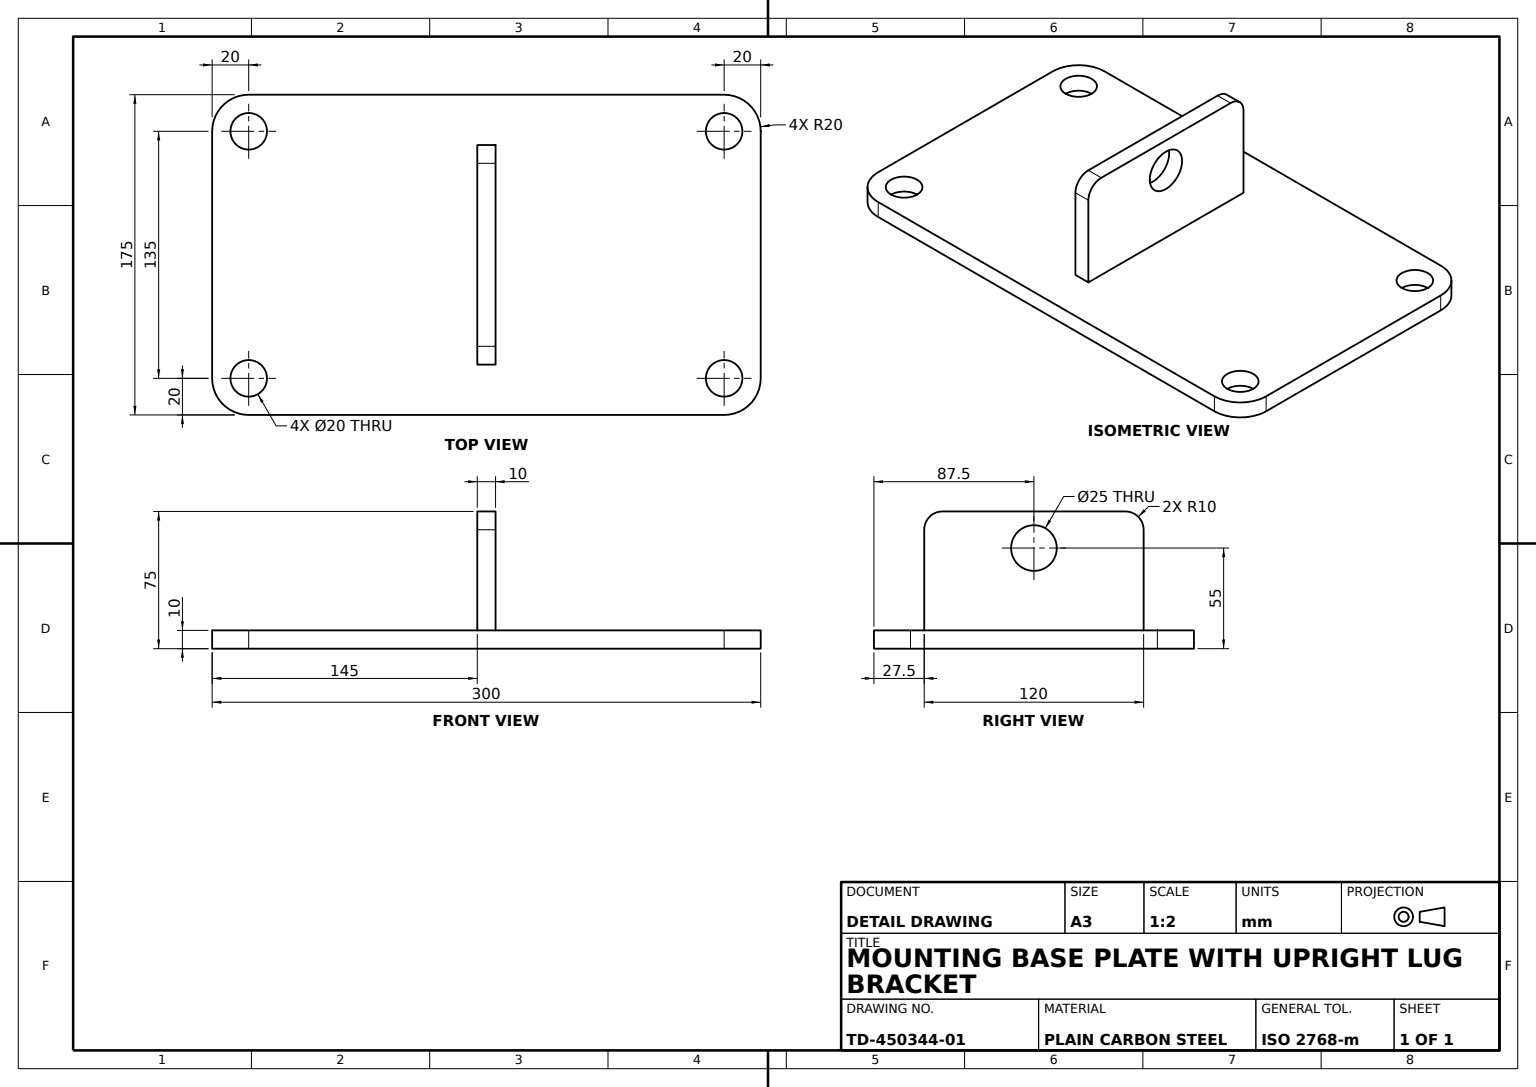
from build123d import *

# Parameters (mm, degrees)
BASE_PLATE_DEPTH          = 10
MOUNTING_HOLES_SKETCH_R   = 10
MOUNTING_HOLES_4X_DEPTH   = 10
UPRIGHT_TAB_SKETCH_W      = 10
UPRIGHT_TAB_SKETCH_H      = 120
UPRIGHT_TAB_DEPTH         = 65
TAB_CORNER_FILLET_1_R10_R = 10
TAB_CORNER_FILLET_2_R10_R = 10
TAB_HOLE_SKETCH_R         = 12.5
TAB_HOLE_DEPTH            = 65


with BuildPart() as part:
    # Base Plate Sketch → Base Plate (new body)
    with BuildSketch(Plane(origin=(0, 0, 0), x_dir=(1, 0, 0), z_dir=(0, 1, 0))):
        with BuildLine():
            Line((-130, -87.5), (130, -87.5))
            ThreePointArc((130, -87.5), (144.142135624, -81.642135624), (150, -67.5))
            Line((150, -67.5), (150, 67.5))
            ThreePointArc((150, 67.5), (144.142135624, 81.642135624), (130, 87.5))
            Line((130, 87.5), (-130, 87.5))
            ThreePointArc((-130, 87.5), (-144.142135624, 81.642135624), (-150, 67.5))
            Line((-150, 67.5), (-150, -67.5))
            ThreePointArc((-150, -67.5), (-144.142135624, -81.642135624), (-130, -87.5))
        make_face()
    extrude(amount=BASE_PLATE_DEPTH)

    # Mounting Holes Sketch → Mounting Holes 4x (cut)
    with BuildSketch(Plane(origin=(0, 10, 0), x_dir=(1, 0, 0), z_dir=(0, 1, 0))):
        with Locations(Location((130, 67.5, 0), (0, 0, 270))):
            Circle(MOUNTING_HOLES_SKETCH_R)
        with Locations(Location((130, -67.5, 0), (0, 0, 270))):
            Circle(MOUNTING_HOLES_SKETCH_R)
        with Locations(Location((-130, 67.5, 0), (0, 0, 270))):
            Circle(MOUNTING_HOLES_SKETCH_R)
        with Locations(Location((-130, -67.5, 0), (0, 0, 270))):
            Circle(MOUNTING_HOLES_SKETCH_R)
    extrude(amount=-MOUNTING_HOLES_4X_DEPTH, mode=Mode.SUBTRACT)

    # Upright Tab Sketch → Upright Tab (add)
    with BuildSketch(Plane(origin=(0, 10, 0), x_dir=(1, 0, 0), z_dir=(0, 1, 0))):
        Rectangle(UPRIGHT_TAB_SKETCH_W, UPRIGHT_TAB_SKETCH_H)
    extrude(amount=UPRIGHT_TAB_DEPTH)

    # Tab Corner Fillet 1 R10
    tab_corner_fillet_1_r10_edges = [part.edges().sort_by_distance(p)[0] for p in [
        (0, 75, 60),
    ]]
    fillet(tab_corner_fillet_1_r10_edges, radius=TAB_CORNER_FILLET_1_R10_R)

    # Tab Corner Fillet 2 R10
    tab_corner_fillet_2_r10_edges = [part.edges().sort_by_distance(p)[0] for p in [
        (0, 75, -60),
    ]]
    fillet(tab_corner_fillet_2_r10_edges, radius=TAB_CORNER_FILLET_2_R10_R)

    # Tab Hole Sketch → Tab Hole (cut)
    with BuildSketch(Plane(origin=(5, 0, 0), x_dir=(0, 0, -1), z_dir=(1, 0, 0))):
        with Locations((0, 55)):
            Circle(TAB_HOLE_SKETCH_R)
    extrude(amount=-TAB_HOLE_DEPTH, mode=Mode.SUBTRACT)


solid = part.part
